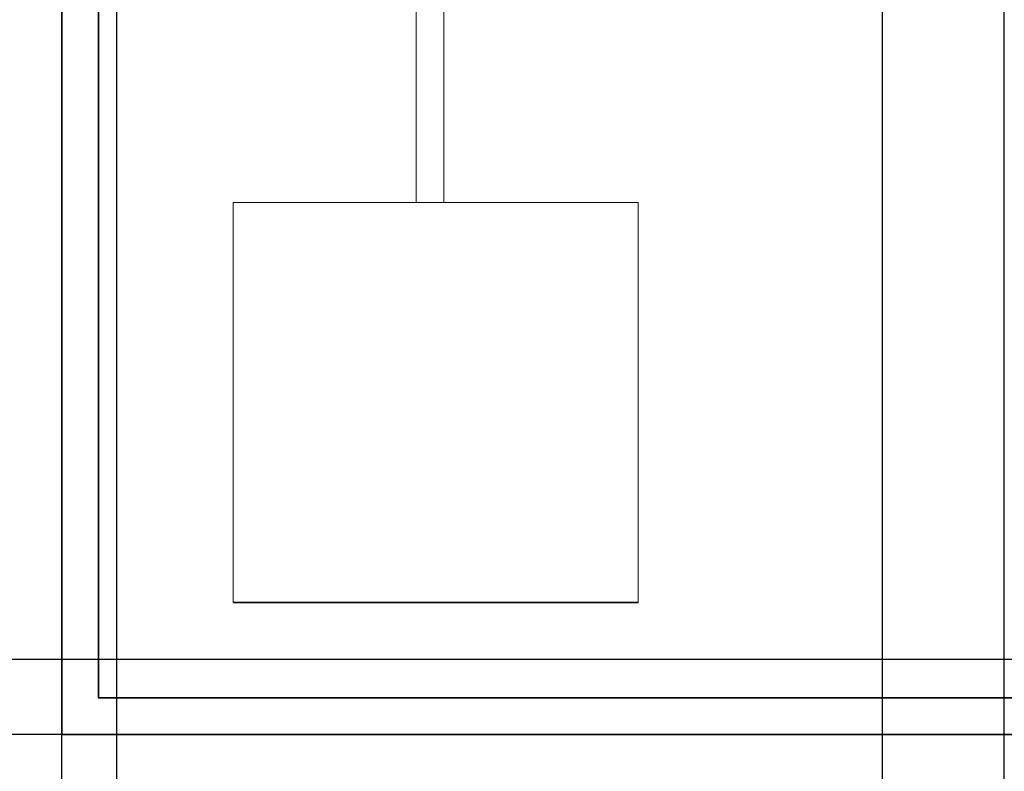
# Model space of a CAD drawing. Units: millimetres. Extents: x 446512 to 447461, y 70395 to 70610.
# Tile 11 of 39: x 446686 to 446699.43, y 70472.88 to 70483.13. Entities that reach past the tile are written whole.
import ezdxf

# ---------------------------------------------------------------- set-up
doc = ezdxf.new("R2010")
doc.units = ezdxf.units.MM
for name, color, linetype, lineweight in [('A-ANNO-DIMS', 2, 'Continuous', 18), ('A-CONS', 9, 'Continuous', 13), ('A-FURN', 7, 'Continuous', 35), ('A-FURN-DECO', 8, 'Continuous', 13)]:
    doc.layers.add(name, color=color, linetype=linetype, lineweight=lineweight)
doc.styles.get("Standard").update_dxf_attribs({"font": 'arial.ttf'})
doc.dimstyles.get("Standard").update_dxf_attribs({"dimtxt": 0.18, "dimasz": 0.18, "dimexe": 0.18, "dimexo": 0.0625, "dimgap": 0.09, "dimtad": 0, "dimtih": 1, "dimtoh": 1, "dimdec": 4, "dimzin": 0, "dimdsep": 46, "dimtxsty": 'Standard', "dimcen": 0.09, "dimadec": 0, "dimazin": 0, "dimtfac": 1, "dimtdec": 4, "dimtofl": 0, "dimtmove": 0, "dimatfit": 3, "dimfxl": 1, "dimtolj": 1, "dimtzin": 0, "dimarcsym": 0})

# ---------------------------------------------------------------- blocks, each defined once
blk = doc.blocks.new('*D20')
at = {"layer": 'A-ANNO-DIMS', "color": 0, "lineweight": -2, "transparency": 16777216}
for p, q in [((446686.51, 70473.382), (446678.043, 70473.382)), ((446678.223, 70473.202), (446678.223, 70463.563)), ((446678.223, 70453.562), (446678.223, 70463.2)), ((446686.51, 70453.382), (446678.043, 70453.382))]:
    blk.add_line(p, q, dxfattribs=at)
at = {"layer": 'A-ANNO-DIMS', "color": 0, "transparency": 16777216}
for points in [[(446678.193, 70473.202), (446678.253, 70473.202), (446678.223, 70473.382)], [(446678.193, 70453.562), (446678.253, 70453.562), (446678.223, 70453.382)]]:
    blk.add_solid(points, dxfattribs=at)
at = {"layer": 'Defpoints', "color": 0, "transparency": 16777216}
for p in [(446678.223, 70473.382), (446686.573, 70473.382), (446686.573, 70453.382)]:
    blk.add_point(p, dxfattribs=at)
at = {"layer": 'A-ANNO-DIMS', "color": 0, "transparency": 16777216, "insert": (446678.223, 70463.382), "char_height": 0.18, "attachment_point": 5}
blk.add_mtext('\\A1;20', dxfattribs=at)
blk = doc.blocks.new('*D21')
at = {"layer": 'A-ANNO-DIMS', "color": 0, "lineweight": -2, "transparency": 16777216}
for p, q in [((446686.51, 70493.382), (446678.043, 70493.382)), ((446678.223, 70493.202), (446678.223, 70483.563)), ((446678.223, 70473.562), (446678.223, 70483.2)), ((446686.51, 70473.382), (446678.043, 70473.382))]:
    blk.add_line(p, q, dxfattribs=at)
at = {"layer": 'A-ANNO-DIMS', "color": 0, "transparency": 16777216}
for points in [[(446678.193, 70493.202), (446678.253, 70493.202), (446678.223, 70493.382)], [(446678.193, 70473.562), (446678.253, 70473.562), (446678.223, 70473.382)]]:
    blk.add_solid(points, dxfattribs=at)
at = {"layer": 'Defpoints', "color": 0, "transparency": 16777216}
for p in [(446678.223, 70493.382), (446686.573, 70493.382), (446686.573, 70473.382)]:
    blk.add_point(p, dxfattribs=at)
at = {"layer": 'A-ANNO-DIMS', "color": 0, "transparency": 16777216, "insert": (446678.223, 70483.382), "char_height": 0.18, "attachment_point": 5}
blk.add_mtext('\\A1;20', dxfattribs=at)
blk = doc.blocks.new('*D32')
at = {"layer": 'A-ANNO-DIMS', "color": 0, "lineweight": -2, "transparency": 16777216}
for p, q in [((446730.76, 70474.405), (446678.043, 70474.405)), ((446678.223, 70474.225), (446678.223, 70474.075)), ((446678.223, 70473.562), (446678.223, 70473.711)), ((446728.946, 70473.382), (446678.043, 70473.382))]:
    blk.add_line(p, q, dxfattribs=at)
at = {"layer": 'A-ANNO-DIMS', "color": 0, "transparency": 16777216}
for points in [[(446678.193, 70474.225), (446678.253, 70474.225), (446678.223, 70474.405)], [(446678.193, 70473.562), (446678.253, 70473.562), (446678.223, 70473.382)]]:
    blk.add_solid(points, dxfattribs=at)
at = {"layer": 'Defpoints', "color": 0, "transparency": 16777216}
for p in [(446730.822, 70474.405), (446678.223, 70473.382), (446729.008, 70473.382)]:
    blk.add_point(p, dxfattribs=at)
at = {"layer": 'A-ANNO-DIMS', "color": 0, "transparency": 16777216, "insert": (446678.223, 70473.893), "char_height": 0.18, "attachment_point": 5}
blk.add_mtext('\\A1;1.02', dxfattribs=at)
blk = doc.blocks.new('*D37')
at = {"layer": 'A-ANNO-DIMS', "color": 0, "lineweight": -2, "transparency": 16777216}
for p, q in [((446686.572846, 70433.44405), (446686.572846, 70578.17492)), ((446687.323552, 70428.838404), (446687.323552, 70578.17492)), ((446686.392846, 70577.99492), (446686.212846, 70577.99492)), ((446687.503552, 70577.99492), (446687.683552, 70577.99492))]:
    blk.add_line(p, q, dxfattribs=at)
at = {"layer": 'A-ANNO-DIMS', "color": 0, "transparency": 16777216}
for points in [[(446686.392846, 70578.02492), (446686.392846, 70577.96492), (446686.572846, 70577.99492)], [(446687.503552, 70578.02492), (446687.503552, 70577.96492), (446687.323552, 70577.99492)]]:
    blk.add_solid(points, dxfattribs=at)
at = {"layer": 'Defpoints', "color": 0, "transparency": 16777216}
for p in [(446687.323552, 70577.99492), (446686.572846, 70433.38155), (446687.323552, 70428.775904)]:
    blk.add_point(p, dxfattribs=at)
at = {"layer": 'A-ANNO-DIMS', "color": 0, "transparency": 16777216, "insert": (446686.948199, 70577.99492), "char_height": 0.18, "attachment_point": 5}
blk.add_mtext('\\A1;0.75', dxfattribs=at)
blk = doc.blocks.new('*D38')
at = {"layer": 'A-ANNO-DIMS', "color": 0, "lineweight": -2, "transparency": 16777216}
for p, q in [((446687.323552, 70428.838404), (446687.323552, 70578.17492)), ((446697.765686, 70428.838404), (446697.765686, 70578.17492)), ((446687.503552, 70577.99492), (446692.090383, 70577.99492)), ((446697.585686, 70577.99492), (446692.998855, 70577.99492))]:
    blk.add_line(p, q, dxfattribs=at)
at = {"layer": 'A-ANNO-DIMS', "color": 0, "transparency": 16777216}
for points in [[(446687.503552, 70578.02492), (446687.503552, 70577.96492), (446687.323552, 70577.99492)], [(446697.585686, 70578.02492), (446697.585686, 70577.96492), (446697.765686, 70577.99492)]]:
    blk.add_solid(points, dxfattribs=at)
at = {"layer": 'Defpoints', "color": 0, "transparency": 16777216}
for p in [(446697.765686, 70577.99492), (446687.323552, 70428.775904), (446697.765686, 70428.775904)]:
    blk.add_point(p, dxfattribs=at)
at = {"layer": 'A-ANNO-DIMS', "color": 0, "transparency": 16777216, "insert": (446692.544619, 70577.99492), "char_height": 0.18, "attachment_point": 5}
blk.add_mtext('\\A1;10.442', dxfattribs=at)
blk = doc.blocks.new('*D39')
at = {"layer": 'A-ANNO-DIMS', "color": 0, "lineweight": -2, "transparency": 16777216}
for p, q in [((446697.766, 70428.838), (446697.766, 70578.175)), ((446699.429, 70433.444), (446699.429, 70578.175)), ((446697.946, 70577.995), (446698.212, 70577.995)), ((446699.249, 70577.995), (446698.982, 70577.995))]:
    blk.add_line(p, q, dxfattribs=at)
at = {"layer": 'A-ANNO-DIMS', "color": 0, "transparency": 16777216}
for points in [[(446697.946, 70578.025), (446697.946, 70577.965), (446697.766, 70577.995)], [(446699.249, 70578.025), (446699.249, 70577.965), (446699.429, 70577.995)]]:
    blk.add_solid(points, dxfattribs=at)
at = {"layer": 'Defpoints', "color": 0, "transparency": 16777216}
for p in [(446699.429, 70577.995), (446699.429, 70433.382), (446697.766, 70428.776)]:
    blk.add_point(p, dxfattribs=at)
at = {"layer": 'A-ANNO-DIMS', "color": 0, "transparency": 16777216, "insert": (446698.597, 70577.995), "char_height": 0.18, "attachment_point": 5}
blk.add_mtext('\\A1;1.663', dxfattribs=at)

msp = doc.modelspace()

# ---------------------------------------------------------------- linework, layer by layer
at = {"layer": 'A-CONS'}
msp.add_point((446686.5728, 70473.3815), dxfattribs=at)
at = {"layer": 'A-FURN'}
for p, q in [((446686.5728, 70473.3815), (446686.5728, 70493.3815)), ((446688.9102, 70475.1818), (446694.4331, 70475.1818)), ((446686.5728, 70473.3815), (446746.5728, 70473.3815))]:
    msp.add_line(p, q, dxfattribs=at)
for points in [[(446686.5728, 70493.3815), (446729.0084, 70493.3815), (446729.0084, 70473.3815), (446686.5728, 70473.3815)], [(446687.0728, 70492.8815), (446728.5084, 70492.8815), (446728.5084, 70473.8815), (446687.0728, 70473.8815)]]:
    msp.add_lwpolyline(points, close=True, dxfattribs=at)
at = {"layer": 'A-FURN-DECO'}
for p, q in [((446691.4074, 70480.6395), (446691.4074, 70483.917)), ((446691.7829, 70480.6395), (446691.7829, 70483.7752)), ((446688.9102, 70475.1818), (446688.9102, 70480.6395)), ((446688.9102, 70480.6395), (446691.4074, 70480.6395)), ((446691.7829, 70480.6395), (446691.4074, 70480.6395)), ((446691.7829, 70480.6395), (446694.4331, 70480.6395)), ((446694.4331, 70475.1818), (446694.4331, 70480.6395))]:
    msp.add_line(p, q, dxfattribs=at)

# ---------------------------------------------------------------- dimensions: what is measured, and where the dimension line sits
at = {"layer": 'A-ANNO-DIMS'}
for base, p1, p2, override, picture, middle in [((446687.3236, 70577.9949), (446686.5728, 70433.3816), (446687.3236, 70428.7759), {"dimdec": 2, "dimlfac": 1, "dimrnd": 0, "dimzin": 0, "dimdsep": 46, "dimlunit": 2}, '*D37', (446686.9482, 70577.9949)), ((446697.7657, 70577.9949), (446687.3236, 70428.7759), (446697.7657, 70428.7759), {"dimdec": 3, "dimlfac": 1, "dimrnd": 0, "dimzin": 0, "dimdsep": 46, "dimlunit": 2}, '*D38', (446692.5446, 70577.9949)), ((446699.4288, 70577.9949), (446697.7657, 70428.7759), (446699.4288, 70433.3816), {"dimdec": 3, "dimlfac": 1, "dimrnd": 0, "dimzin": 0, "dimdsep": 46, "dimlunit": 2}, '*D39', (446698.5973, 70577.9949))]:
    dim = msp.add_linear_dim(base=base, p1=p1, p2=p2, dimstyle='Standard', override=override, dxfattribs=at)
    dim.commit()
    dim.dimension.update_dxf_attribs({"geometry": picture, "text_midpoint": middle})
for base, p1, p2, override, picture, middle in [((446678.2228, 70493.3815), (446686.5728, 70473.3815), (446686.5728, 70493.3815), {"dimdec": 0, "dimlfac": 1, "dimrnd": 0, "dimzin": 0, "dimdsep": 46, "dimlunit": 2}, '*D21', (446678.2228, 70483.3815)), ((446678.2228, 70473.3815), (446730.8224, 70474.4047), (446729.0084, 70473.3815), {"dimdec": 2, "dimlfac": 1, "dimrnd": 0, "dimzin": 0, "dimdsep": 46, "dimlunit": 2}, '*D32', (446678.2228, 70473.8931)), ((446678.2228, 70473.3815), (446686.5728, 70453.3816), (446686.5728, 70473.3815), {"dimdec": 0, "dimlfac": 1, "dimrnd": 0, "dimzin": 0, "dimdsep": 46, "dimlunit": 2}, '*D20', (446678.2228, 70463.3815))]:
    dim = msp.add_linear_dim(base=base, p1=p1, p2=p2, angle=90, dimstyle='Standard', override=override, dxfattribs=at)
    dim.commit()
    dim.dimension.update_dxf_attribs({"geometry": picture, "text_midpoint": middle})

doc.saveas('drawing.dxf')
